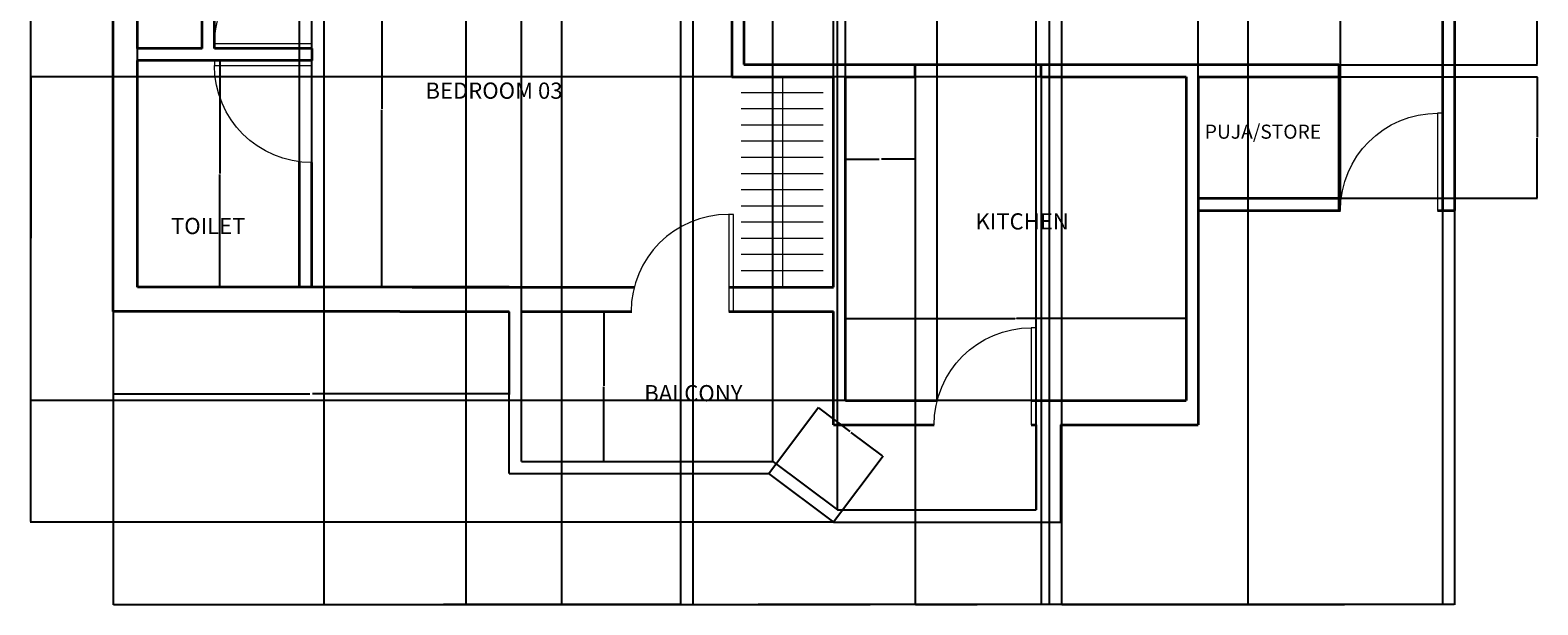
# Model space of a CAD drawing. Units: inches. Extents: x -83 to 475, y -99 to 539.
# Tile 1 of 3: x -83 to 475, y -99 to 114. Entities that reach past the tile are written whole.
import ezdxf

# ---------------------------------------------------------------- set-up
doc = ezdxf.new("R2010")
doc.units = ezdxf.units.IN
doc.header["$LTSCALE"] = 0.5
doc.header["$MEASUREMENT"] = 0
for name, color, linetype, lineweight in [('A-ANNO-DIMS', 2, 'Continuous', 18), ('A-AREA-IDEN', 7, 'Continuous', 18), ('A-DOOR', 3, 'Continuous', 18), ('A-FURN', 8, 'Continuous', 13), ('A-WALL', 7, 'Continuous', 35), ('A-WALL-PRPT', 7, 'Continuous', 25)]:
    doc.layers.add(name, color=color, linetype=linetype, lineweight=lineweight)
doc.styles.get("Standard").update_dxf_attribs({"font": 'arial.ttf'})
doc.dimstyles.get("Standard").update_dxf_attribs({"dimtxt": 0.18, "dimasz": 0.18, "dimexe": 0.18, "dimexo": 0.0625, "dimgap": 0.09, "dimtad": 0, "dimtih": 1, "dimtoh": 1, "dimdec": 4, "dimzin": 0, "dimdsep": 46, "dimtxsty": 'Standard', "dimcen": 0.09, "dimadec": 0, "dimazin": 0, "dimtfac": 1, "dimtdec": 4, "dimtofl": 0, "dimtmove": 0, "dimatfit": 3, "dimfxl": 1, "dimtolj": 1, "dimtzin": 0, "dimarcsym": 0})

# ---------------------------------------------------------------- blocks, each defined once
blk = doc.blocks.new('DOOR-SWING-36')
blk.add_lwpolyline([(1.78, 0), (0, 0), (0, 36.03), (1.78, 36.03)], close=True)
blk.add_arc((1.78, 0), 36, 0, 90)
blk = doc.blocks.new('*D14')
at = {"layer": 'A-ANNO-DIMS', "color": 0, "lineweight": -2, "transparency": 16777216}
for p, q in [((444.04, 47.05), (444.04, -99.07)), ((-52.46, 9.55), (-52.46, -99.07)), ((-52.28, -98.89), (195.39, -98.89)), ((443.86, -98.89), (196.19, -98.89))]:
    blk.add_line(p, q, dxfattribs=at)
at = {"layer": 'A-ANNO-DIMS', "color": 0, "transparency": 16777216}
for points in [[(-52.28, -98.86), (-52.28, -98.92), (-52.46, -98.89)], [(443.86, -98.86), (443.86, -98.92), (444.04, -98.89)]]:
    blk.add_solid(points, dxfattribs=at)
at = {"layer": 'Defpoints', "color": 0, "transparency": 16777216}
for p in [(444.04, 47.11), (-52.46, 9.61), (444.04, -98.89)]:
    blk.add_point(p, dxfattribs=at)
at = {"layer": 'A-ANNO-DIMS', "color": 0, "transparency": 16777216, "insert": (195.79, -98.89), "char_height": 0.18, "attachment_point": 5}
blk.add_mtext('\\A1;496.5', dxfattribs=at)
blk = doc.blocks.new('*D15')
at = {"layer": 'A-ANNO-DIMS', "color": 0, "lineweight": -2, "transparency": 16777216}
for p, q in [((73.48, 492.61), (-83.14, 492.61)), ((-82.96, 492.43), (-82.96, 212.3)), ((-82.96, -68.21), (-82.96, 211.93)), ((214.1, -68.39), (-83.14, -68.39))]:
    blk.add_line(p, q, dxfattribs=at)
at = {"layer": 'A-ANNO-DIMS', "color": 0, "transparency": 16777216}
for points in [[(-82.99, 492.43), (-82.93, 492.43), (-82.96, 492.61)], [(-82.99, -68.21), (-82.93, -68.21), (-82.96, -68.39)]]:
    blk.add_solid(points, dxfattribs=at)
at = {"layer": 'Defpoints', "color": 0, "transparency": 16777216}
for p in [(-82.96, 492.61), (73.54, 492.61), (214.16, -68.39)]:
    blk.add_point(p, dxfattribs=at)
at = {"layer": 'A-ANNO-DIMS', "color": 0, "transparency": 16777216, "insert": (-82.96, 212.11), "char_height": 0.18, "attachment_point": 5}
blk.add_mtext('\\A1;561', dxfattribs=at)
blk = doc.blocks.new('*D16')
at = {"layer": 'A-ANNO-DIMS', "color": 0, "lineweight": -2, "transparency": 16777216}
for p, q in [((78.04, 488.05), (78.04, -99.07)), ((294.04, 488.05), (294.04, -99.07)), ((78.22, -98.89), (185.75, -98.89)), ((293.86, -98.89), (186.33, -98.89))]:
    blk.add_line(p, q, dxfattribs=at)
at = {"layer": 'A-ANNO-DIMS', "color": 0, "transparency": 16777216}
for points in [[(78.22, -98.86), (78.22, -98.92), (78.04, -98.89)], [(293.86, -98.86), (293.86, -98.92), (294.04, -98.89)]]:
    blk.add_solid(points, dxfattribs=at)
at = {"layer": 'Defpoints', "color": 0, "transparency": 16777216}
for p in [(78.04, 488.11), (294.04, 488.11), (294.04, -98.89)]:
    blk.add_point(p, dxfattribs=at)
at = {"layer": 'A-ANNO-DIMS', "color": 0, "transparency": 16777216, "insert": (186.04, -98.89), "char_height": 0.18, "attachment_point": 5}
blk.add_mtext('\\A1;216', dxfattribs=at)
blk = doc.blocks.new('*D19')
at = {"layer": 'A-ANNO-DIMS', "color": 0, "lineweight": -2, "transparency": 16777216}
for p, q in [((25.54, 375.55), (25.54, -99.07)), ((157.54, 375.55), (157.54, -99.07)), ((25.72, -98.89), (91.26, -98.89)), ((157.36, -98.89), (91.82, -98.89))]:
    blk.add_line(p, q, dxfattribs=at)
at = {"layer": 'A-ANNO-DIMS', "color": 0, "transparency": 16777216}
for points in [[(25.72, -98.86), (25.72, -98.92), (25.54, -98.89)], [(157.36, -98.86), (157.36, -98.92), (157.54, -98.89)]]:
    blk.add_solid(points, dxfattribs=at)
at = {"layer": 'Defpoints', "color": 0, "transparency": 16777216}
for p in [(25.54, 375.61), (157.54, 375.61), (157.54, -98.89)]:
    blk.add_point(p, dxfattribs=at)
at = {"layer": 'A-ANNO-DIMS', "color": 0, "transparency": 16777216, "insert": (91.54, -98.89), "char_height": 0.18, "attachment_point": 5}
blk.add_mtext('\\A1;132', dxfattribs=at)
blk = doc.blocks.new('*D20')
at = {"layer": 'A-ANNO-DIMS', "color": 0, "lineweight": -2, "transparency": 16777216}
for p, q in [((162.04, 375.55), (162.04, -99.07)), ((294.04, 357.55), (294.04, -99.07)), ((162.22, -98.89), (227.76, -98.89)), ((293.86, -98.89), (228.32, -98.89))]:
    blk.add_line(p, q, dxfattribs=at)
at = {"layer": 'A-ANNO-DIMS', "color": 0, "transparency": 16777216}
for points in [[(162.22, -98.86), (162.22, -98.92), (162.04, -98.89)], [(293.86, -98.86), (293.86, -98.92), (294.04, -98.89)]]:
    blk.add_solid(points, dxfattribs=at)
at = {"layer": 'Defpoints', "color": 0, "transparency": 16777216}
for p in [(162.04, 375.61), (294.04, 357.61), (294.04, -98.89)]:
    blk.add_point(p, dxfattribs=at)
at = {"layer": 'A-ANNO-DIMS', "color": 0, "transparency": 16777216, "insert": (228.04, -98.89), "char_height": 0.18, "attachment_point": 5}
blk.add_mtext('\\A1;132', dxfattribs=at)
blk = doc.blocks.new('*D27')
at = {"layer": 'A-ANNO-DIMS', "color": 0, "lineweight": -2, "transparency": 16777216}
for p, q in [((367.54, 345.55), (367.54, -99.07)), ((439.54, 345.55), (439.54, -99.07)), ((367.72, -98.89), (403.32, -98.89)), ((439.36, -98.89), (403.76, -98.89))]:
    blk.add_line(p, q, dxfattribs=at)
at = {"layer": 'A-ANNO-DIMS', "color": 0, "transparency": 16777216}
for points in [[(367.72, -98.86), (367.72, -98.92), (367.54, -98.89)], [(439.36, -98.86), (439.36, -98.92), (439.54, -98.89)]]:
    blk.add_solid(points, dxfattribs=at)
at = {"layer": 'Defpoints', "color": 0, "transparency": 16777216}
for p in [(367.54, 345.61), (439.54, 345.61), (439.54, -98.89)]:
    blk.add_point(p, dxfattribs=at)
at = {"layer": 'A-ANNO-DIMS', "color": 0, "transparency": 16777216, "insert": (403.54, -98.89), "char_height": 0.18, "attachment_point": 5}
blk.add_mtext('\\A1;72', dxfattribs=at)
blk = doc.blocks.new('*D33')
at = {"layer": 'A-ANNO-DIMS', "color": 0, "lineweight": -2, "transparency": 16777216}
for p, q in [((25.54, 215.05), (25.54, -99.07)), ((113.54, 215.05), (113.54, -99.07)), ((25.72, -98.89), (69.32, -98.89)), ((113.36, -98.89), (69.76, -98.89))]:
    blk.add_line(p, q, dxfattribs=at)
at = {"layer": 'A-ANNO-DIMS', "color": 0, "transparency": 16777216}
for points in [[(25.72, -98.86), (25.72, -98.92), (25.54, -98.89)], [(113.36, -98.86), (113.36, -98.92), (113.54, -98.89)]]:
    blk.add_solid(points, dxfattribs=at)
at = {"layer": 'Defpoints', "color": 0, "transparency": 16777216}
for p in [(25.54, 215.11), (113.54, 215.11), (113.54, -98.89)]:
    blk.add_point(p, dxfattribs=at)
at = {"layer": 'A-ANNO-DIMS', "color": 0, "transparency": 16777216, "insert": (69.54, -98.89), "char_height": 0.18, "attachment_point": 5}
blk.add_mtext('\\A1;88', dxfattribs=at)
blk = doc.blocks.new('*D35')
at = {"layer": 'A-ANNO-DIMS', "color": 0, "lineweight": -2, "transparency": 16777216}
for p, q in [((21.04, 18.68), (21.04, 523.29)), ((21.22, 523.11), (117.15, 523.11)), ((213.98, 523.11), (118.05, 523.11)), ((214.16, 18.68), (214.16, 523.29))]:
    blk.add_line(p, q, dxfattribs=at)
at = {"layer": 'A-ANNO-DIMS', "color": 0, "transparency": 16777216}
for points in [[(21.22, 523.14), (21.22, 523.08), (21.04, 523.11)], [(213.98, 523.14), (213.98, 523.08), (214.16, 523.11)]]:
    blk.add_solid(points, dxfattribs=at)
at = {"layer": 'Defpoints', "color": 0, "transparency": 16777216}
for p in [(214.16, 523.11), (21.04, 18.61), (214.16, 18.61)]:
    blk.add_point(p, dxfattribs=at)
at = {"layer": 'A-ANNO-DIMS', "color": 0, "transparency": 16777216, "insert": (117.6, 523.11), "char_height": 0.18, "attachment_point": 5}
blk.add_mtext('\\A1;193.12', dxfattribs=at)
blk = doc.blocks.new('*D36')
at = {"layer": 'A-ANNO-DIMS', "color": 0, "lineweight": -2, "transparency": 16777216}
for p, q in [((16.6, 150.61), (47.22, 150.61)), ((47.04, 150.43), (47.04, 84.8)), ((47.04, 18.79), (47.04, 84.43)), ((16.6, 18.61), (47.22, 18.61))]:
    blk.add_line(p, q, dxfattribs=at)
at = {"layer": 'A-ANNO-DIMS', "color": 0, "transparency": 16777216}
for points in [[(47.01, 150.43), (47.07, 150.43), (47.04, 150.61)], [(47.01, 18.79), (47.07, 18.79), (47.04, 18.61)]]:
    blk.add_solid(points, dxfattribs=at)
at = {"layer": 'Defpoints', "color": 0, "transparency": 16777216}
for p in [(16.54, 150.61), (16.54, 18.61), (47.04, 18.61)]:
    blk.add_point(p, dxfattribs=at)
at = {"layer": 'A-ANNO-DIMS', "color": 0, "transparency": 16777216, "insert": (47.04, 84.61), "char_height": 0.18, "attachment_point": 5}
blk.add_mtext('\\A1;132', dxfattribs=at)
blk = doc.blocks.new('*D37')
at = {"layer": 'A-ANNO-DIMS', "color": 0, "lineweight": -2, "transparency": 16777216}
for p, q in [((-43.46, 18.68), (-43.46, 523.29)), ((-43.28, 523.11), (-13.68, 523.11)), ((16.36, 523.11), (-13.24, 523.11)), ((16.54, 18.68), (16.54, 523.29))]:
    blk.add_line(p, q, dxfattribs=at)
at = {"layer": 'A-ANNO-DIMS', "color": 0, "transparency": 16777216}
for points in [[(-43.28, 523.14), (-43.28, 523.08), (-43.46, 523.11)], [(16.36, 523.14), (16.36, 523.08), (16.54, 523.11)]]:
    blk.add_solid(points, dxfattribs=at)
at = {"layer": 'Defpoints', "color": 0, "transparency": 16777216}
for p in [(16.54, 523.11), (-43.46, 18.61), (16.54, 18.61)]:
    blk.add_point(p, dxfattribs=at)
at = {"layer": 'A-ANNO-DIMS', "color": 0, "transparency": 16777216, "insert": (-13.46, 523.11), "char_height": 0.18, "attachment_point": 5}
blk.add_mtext('\\A1;60', dxfattribs=at)
blk = doc.blocks.new('*D38')
at = {"layer": 'A-ANNO-DIMS', "color": 0, "lineweight": -2, "transparency": 16777216}
for p, q in [((-43.4, 102.61), (-12.78, 102.61)), ((-12.96, 102.43), (-12.96, 60.8)), ((-12.96, 18.79), (-12.96, 60.43)), ((-43.4, 18.61), (-12.78, 18.61))]:
    blk.add_line(p, q, dxfattribs=at)
at = {"layer": 'A-ANNO-DIMS', "color": 0, "transparency": 16777216}
for points in [[(-12.99, 102.43), (-12.93, 102.43), (-12.96, 102.61)], [(-12.99, 18.79), (-12.93, 18.79), (-12.96, 18.61)]]:
    blk.add_solid(points, dxfattribs=at)
at = {"layer": 'Defpoints', "color": 0, "transparency": 16777216}
for p in [(-43.46, 102.61), (-43.46, 18.61), (-12.96, 18.61)]:
    blk.add_point(p, dxfattribs=at)
at = {"layer": 'A-ANNO-DIMS', "color": 0, "transparency": 16777216, "insert": (-12.96, 60.61), "char_height": 0.18, "attachment_point": 5}
blk.add_mtext('\\A1;84', dxfattribs=at)
blk = doc.blocks.new('*D39')
at = {"layer": 'A-ANNO-DIMS', "color": 0, "lineweight": -2, "transparency": 16777216}
for p, q in [((218.66, -23.32), (218.66, 7.29)), ((218.84, 7.11), (281.38, 7.11)), ((344.48, 7.11), (281.94, 7.11)), ((344.66, -23.32), (344.66, 7.29))]:
    blk.add_line(p, q, dxfattribs=at)
at = {"layer": 'A-ANNO-DIMS', "color": 0, "transparency": 16777216}
for points in [[(218.84, 7.14), (218.84, 7.08), (218.66, 7.11)], [(344.48, 7.14), (344.48, 7.08), (344.66, 7.11)]]:
    blk.add_solid(points, dxfattribs=at)
at = {"layer": 'Defpoints', "color": 0, "transparency": 16777216}
for p in [(344.66, 7.11), (218.66, -23.39), (344.66, -23.39)]:
    blk.add_point(p, dxfattribs=at)
at = {"layer": 'A-ANNO-DIMS', "color": 0, "transparency": 16777216, "insert": (281.66, 7.11), "char_height": 0.18, "attachment_point": 5}
blk.add_mtext('\\A1;126', dxfattribs=at)
blk = doc.blocks.new('*D40')
at = {"layer": 'A-ANNO-DIMS', "color": 0, "lineweight": -2, "transparency": 16777216}
for p, q in [((344.6, 96.61), (-83.14, 96.61)), ((-82.96, 96.43), (-82.96, 36.8)), ((-82.96, -23.21), (-82.96, 36.43)), ((344.6, -23.39), (-83.14, -23.39))]:
    blk.add_line(p, q, dxfattribs=at)
at = {"layer": 'A-ANNO-DIMS', "color": 0, "transparency": 16777216}
for points in [[(-82.99, 96.43), (-82.93, 96.43), (-82.96, 96.61)], [(-82.99, -23.21), (-82.93, -23.21), (-82.96, -23.39)]]:
    blk.add_solid(points, dxfattribs=at)
at = {"layer": 'Defpoints', "color": 0, "transparency": 16777216}
for p in [(-82.96, 96.61), (344.66, 96.61), (344.66, -23.39)]:
    blk.add_point(p, dxfattribs=at)
at = {"layer": 'A-ANNO-DIMS', "color": 0, "transparency": 16777216, "insert": (-82.96, 36.61), "char_height": 0.18, "attachment_point": 5}
blk.add_mtext('\\A1;120', dxfattribs=at)
blk = doc.blocks.new('*D41')
at = {"layer": 'A-ANNO-DIMS', "color": 0, "lineweight": -2, "transparency": 16777216}
for p, q in [((349.16, 51.68), (349.16, 523.29)), ((349.34, 523.11), (375.13, 523.11)), ((401.58, 523.11), (375.78, 523.11)), ((401.76, 51.68), (401.76, 523.29))]:
    blk.add_line(p, q, dxfattribs=at)
at = {"layer": 'A-ANNO-DIMS', "color": 0, "transparency": 16777216}
for points in [[(349.34, 523.14), (349.34, 523.08), (349.16, 523.11)], [(401.58, 523.14), (401.58, 523.08), (401.76, 523.11)]]:
    blk.add_solid(points, dxfattribs=at)
at = {"layer": 'Defpoints', "color": 0, "transparency": 16777216}
for p in [(401.76, 523.11), (349.16, 51.61), (401.76, 51.61)]:
    blk.add_point(p, dxfattribs=at)
at = {"layer": 'A-ANNO-DIMS', "color": 0, "transparency": 16777216, "insert": (375.46, 523.11), "char_height": 0.18, "attachment_point": 5}
blk.add_mtext('\\A1;52.6', dxfattribs=at)
blk = doc.blocks.new('*D42')
at = {"layer": 'A-ANNO-DIMS', "color": 0, "lineweight": -2, "transparency": 16777216}
for p, q in [((401.22, 96.61), (474.72, 96.61)), ((474.54, 96.43), (474.54, 74.3)), ((474.54, 51.79), (474.54, 73.93)), ((401.82, 51.61), (474.72, 51.61))]:
    blk.add_line(p, q, dxfattribs=at)
at = {"layer": 'A-ANNO-DIMS', "color": 0, "transparency": 16777216}
for points in [[(474.51, 96.43), (474.57, 96.43), (474.54, 96.61)], [(474.51, 51.79), (474.57, 51.79), (474.54, 51.61)]]:
    blk.add_solid(points, dxfattribs=at)
at = {"layer": 'Defpoints', "color": 0, "transparency": 16777216}
for p in [(401.16, 96.61), (474.54, 96.61), (401.76, 51.61)]:
    blk.add_point(p, dxfattribs=at)
at = {"layer": 'A-ANNO-DIMS', "color": 0, "transparency": 16777216, "insert": (474.54, 74.11), "char_height": 0.18, "attachment_point": 5}
blk.add_mtext('\\A1;45', dxfattribs=at)
blk = doc.blocks.new('*D43')
at = {"layer": 'A-ANNO-DIMS', "color": 0, "lineweight": -2, "transparency": 16777216}
for p, q in [((180.98, 101.18), (180.98, 523.29)), ((181.16, 523.11), (309.8, 523.11)), ((439.36, 523.11), (310.73, 523.11)), ((439.54, 83.2), (439.54, 523.29))]:
    blk.add_line(p, q, dxfattribs=at)
at = {"layer": 'A-ANNO-DIMS', "color": 0, "transparency": 16777216}
for points in [[(181.16, 523.14), (181.16, 523.08), (180.98, 523.11)], [(439.36, 523.14), (439.36, 523.08), (439.54, 523.11)]]:
    blk.add_solid(points, dxfattribs=at)
at = {"layer": 'Defpoints', "color": 0, "transparency": 16777216}
for p in [(439.54, 523.11), (180.98, 101.11), (439.54, 83.14)]:
    blk.add_point(p, dxfattribs=at)
at = {"layer": 'A-ANNO-DIMS', "color": 0, "transparency": 16777216, "insert": (310.26, 523.11), "char_height": 0.18, "attachment_point": 5}
blk.add_mtext('\\A1;258.56', dxfattribs=at)
blk = doc.blocks.new('*D44')
at = {"layer": 'A-ANNO-DIMS', "color": 0, "lineweight": -2, "transparency": 16777216}
for p, q in [((439.6, 264.61), (474.72, 264.61)), ((474.54, 264.43), (474.54, 183.05)), ((474.54, 101.29), (474.54, 182.68)), ((401.22, 101.11), (474.72, 101.11))]:
    blk.add_line(p, q, dxfattribs=at)
at = {"layer": 'A-ANNO-DIMS', "color": 0, "transparency": 16777216}
for points in [[(474.51, 264.43), (474.57, 264.43), (474.54, 264.61)], [(474.51, 101.29), (474.57, 101.29), (474.54, 101.11)]]:
    blk.add_solid(points, dxfattribs=at)
at = {"layer": 'Defpoints', "color": 0, "transparency": 16777216}
for p in [(439.54, 264.61), (474.54, 264.61), (401.16, 101.11)]:
    blk.add_point(p, dxfattribs=at)
at = {"layer": 'A-ANNO-DIMS', "color": 0, "transparency": 16777216, "insert": (474.54, 182.86), "char_height": 0.18, "attachment_point": 5}
blk.add_mtext('\\A1;163.5', dxfattribs=at)
blk = doc.blocks.new('*D45')
at = {"layer": 'A-ANNO-DIMS', "color": 0, "lineweight": -2, "transparency": 16777216}
for p, q in [((298.54, 264.55), (298.54, -99.07)), ((439.54, 264.55), (439.54, -99.07)), ((298.72, -98.89), (368.78, -98.89)), ((439.36, -98.89), (369.3, -98.89))]:
    blk.add_line(p, q, dxfattribs=at)
at = {"layer": 'A-ANNO-DIMS', "color": 0, "transparency": 16777216}
for points in [[(298.72, -98.86), (298.72, -98.92), (298.54, -98.89)], [(439.36, -98.86), (439.36, -98.92), (439.54, -98.89)]]:
    blk.add_solid(points, dxfattribs=at)
at = {"layer": 'Defpoints', "color": 0, "transparency": 16777216}
for p in [(298.54, 264.61), (439.54, 264.61), (439.54, -98.89)]:
    blk.add_point(p, dxfattribs=at)
at = {"layer": 'A-ANNO-DIMS', "color": 0, "transparency": 16777216, "insert": (369.04, -98.89), "char_height": 0.18, "attachment_point": 5}
blk.add_mtext('\\A1;141', dxfattribs=at)
blk = doc.blocks.new('*D46')
at = {"layer": 'A-ANNO-DIMS', "color": 0, "lineweight": -2, "transparency": 16777216}
for p, q in [((98.72, 9.61), (129.34, 9.61)), ((129.16, 9.43), (129.16, -17.95)), ((129.16, -45.71), (129.16, -18.32)), ((98.72, -45.89), (129.34, -45.89))]:
    blk.add_line(p, q, dxfattribs=at)
at = {"layer": 'A-ANNO-DIMS', "color": 0, "transparency": 16777216}
for points in [[(129.13, 9.43), (129.19, 9.43), (129.16, 9.61)], [(129.13, -45.71), (129.19, -45.71), (129.16, -45.89)]]:
    blk.add_solid(points, dxfattribs=at)
at = {"layer": 'Defpoints', "color": 0, "transparency": 16777216}
for p in [(98.66, 9.61), (98.66, -45.89), (129.16, -45.89)]:
    blk.add_point(p, dxfattribs=at)
at = {"layer": 'A-ANNO-DIMS', "color": 0, "transparency": 16777216, "insert": (129.16, -18.14), "char_height": 0.18, "attachment_point": 5}
blk.add_mtext('\\A1;55.5', dxfattribs=at)
blk = doc.blocks.new('*D47')
at = {"layer": 'A-ANNO-DIMS', "color": 0, "lineweight": -2, "transparency": 16777216}
for p, q in [((98.66, -45.82), (98.66, 523.29)), ((98.84, 523.11), (144.94, 523.11)), ((191.48, 523.11), (145.38, 523.11)), ((191.66, -45.82), (191.66, 523.29))]:
    blk.add_line(p, q, dxfattribs=at)
at = {"layer": 'A-ANNO-DIMS', "color": 0, "transparency": 16777216}
for points in [[(98.84, 523.14), (98.84, 523.08), (98.66, 523.11)], [(191.48, 523.14), (191.48, 523.08), (191.66, 523.11)]]:
    blk.add_solid(points, dxfattribs=at)
at = {"layer": 'Defpoints', "color": 0, "transparency": 16777216}
for p in [(191.66, 523.11), (98.66, -45.89), (191.66, -45.89)]:
    blk.add_point(p, dxfattribs=at)
at = {"layer": 'A-ANNO-DIMS', "color": 0, "transparency": 16777216, "insert": (145.16, 523.11), "char_height": 0.18, "attachment_point": 5}
blk.add_mtext('\\A1;93', dxfattribs=at)
blk = doc.blocks.new('*D48')
at = {"layer": 'A-ANNO-DIMS', "color": 0, "lineweight": -2, "transparency": 16777216}
for p, q in [((215.66, -63.82), (215.66, 523.29)), ((215.84, 523.11), (252.09, 523.11)), ((288.98, 523.11), (252.73, 523.11)), ((289.16, -63.82), (289.16, 523.29))]:
    blk.add_line(p, q, dxfattribs=at)
at = {"layer": 'A-ANNO-DIMS', "color": 0, "transparency": 16777216}
for points in [[(215.84, 523.14), (215.84, 523.08), (215.66, 523.11)], [(288.98, 523.14), (288.98, 523.08), (289.16, 523.11)]]:
    blk.add_solid(points, dxfattribs=at)
at = {"layer": 'Defpoints', "color": 0, "transparency": 16777216}
for p in [(289.16, 523.11), (215.66, -63.89), (289.16, -63.89)]:
    blk.add_point(p, dxfattribs=at)
at = {"layer": 'A-ANNO-DIMS', "color": 0, "transparency": 16777216, "insert": (252.41, 523.11), "char_height": 0.18, "attachment_point": 5}
blk.add_mtext('\\A1;73.5', dxfattribs=at)
blk = doc.blocks.new('*D49')
at = {"layer": 'A-ANNO-DIMS', "color": 0, "lineweight": -2, "transparency": 16777216}
for p, q in [((190.2, -50.34), (208.57, -25.84)), ((208.6, -26.09), (220.24, -34.82)), ((232.32, -43.88), (220.68, -35.15)), ((214.2, -68.34), (232.57, -43.84))]:
    blk.add_line(p, q, dxfattribs=at)
at = {"layer": 'A-ANNO-DIMS', "color": 0, "transparency": 16777216}
for points in [[(208.62, -26.07), (208.59, -26.12), (208.46, -25.99)], [(232.33, -43.85), (232.3, -43.9), (232.46, -43.99)]]:
    blk.add_solid(points, dxfattribs=at)
at = {"layer": 'Defpoints', "color": 0, "transparency": 16777216}
for p in [(232.46, -43.99), (190.16, -50.39), (214.16, -68.39)]:
    blk.add_point(p, dxfattribs=at)
at = {"layer": 'A-ANNO-DIMS', "color": 0, "transparency": 16777216, "insert": (220.46, -34.99), "char_height": 0.18, "attachment_point": 5}
blk.add_mtext('\\A1;30', dxfattribs=at)
blk = doc.blocks.new('*D50')
at = {"layer": 'A-ANNO-DIMS', "color": 0, "lineweight": -2, "transparency": 16777216}
for p, q in [((-52.46, 9.55), (-52.46, -21.07)), ((94.16, 9.55), (94.16, -21.07)), ((-52.28, -20.89), (20.4, -20.89)), ((93.98, -20.89), (21.3, -20.89))]:
    blk.add_line(p, q, dxfattribs=at)
at = {"layer": 'A-ANNO-DIMS', "color": 0, "transparency": 16777216}
for points in [[(-52.28, -20.86), (-52.28, -20.92), (-52.46, -20.89)], [(93.98, -20.86), (93.98, -20.92), (94.16, -20.89)]]:
    blk.add_solid(points, dxfattribs=at)
at = {"layer": 'Defpoints', "color": 0, "transparency": 16777216}
for p in [(-52.46, 9.61), (94.16, 9.61), (-52.46, -20.89)]:
    blk.add_point(p, dxfattribs=at)
at = {"layer": 'A-ANNO-DIMS', "color": 0, "transparency": 16777216, "insert": (20.85, -20.89), "char_height": 0.18, "attachment_point": 5}
blk.add_mtext('\\A1;146.62', dxfattribs=at)
blk = doc.blocks.new('*D58')
at = {"layer": 'A-ANNO-DIMS', "color": 0, "lineweight": -2, "transparency": 16777216}
for p, q in [((218.66, -23.32), (218.66, 523.29)), ((218.84, 523.11), (235.2, 523.11)), ((252.34, 523.11), (235.98, 523.11)), ((252.52, -23.32), (252.52, 523.29))]:
    blk.add_line(p, q, dxfattribs=at)
at = {"layer": 'A-ANNO-DIMS', "color": 0, "transparency": 16777216}
for points in [[(218.84, 523.14), (218.84, 523.08), (218.66, 523.11)], [(252.34, 523.14), (252.34, 523.08), (252.52, 523.11)]]:
    blk.add_solid(points, dxfattribs=at)
at = {"layer": 'Defpoints', "color": 0, "transparency": 16777216}
for p in [(252.52, 523.11), (218.66, -23.39), (252.52, -23.39)]:
    blk.add_point(p, dxfattribs=at)
at = {"layer": 'A-ANNO-DIMS', "color": 0, "transparency": 16777216, "insert": (235.59, 523.11), "char_height": 0.18, "attachment_point": 5}
blk.add_mtext('\\A1;33.86', dxfattribs=at)
blk = doc.blocks.new('*D59')
at = {"layer": 'A-ANNO-DIMS', "color": 0, "lineweight": -2, "transparency": 16777216}
for p, q in [((218.66, 96.55), (218.66, 65.93)), ((244.35, 96.55), (244.35, 65.93)), ((218.84, 66.11), (231.11, 66.11)), ((244.17, 66.11), (231.9, 66.11))]:
    blk.add_line(p, q, dxfattribs=at)
at = {"layer": 'A-ANNO-DIMS', "color": 0, "transparency": 16777216}
for points in [[(218.84, 66.14), (218.84, 66.08), (218.66, 66.11)], [(244.17, 66.14), (244.17, 66.08), (244.35, 66.11)]]:
    blk.add_solid(points, dxfattribs=at)
at = {"layer": 'Defpoints', "color": 0, "transparency": 16777216}
for p in [(218.66, 96.61), (244.35, 96.61), (218.66, 66.11)]:
    blk.add_point(p, dxfattribs=at)
at = {"layer": 'A-ANNO-DIMS', "color": 0, "transparency": 16777216, "insert": (231.51, 66.11), "char_height": 0.18, "attachment_point": 5}
blk.add_mtext('\\A1;25.69', dxfattribs=at)
blk = doc.blocks.new('*D60')
at = {"layer": 'A-ANNO-DIMS', "color": 0, "lineweight": -2, "transparency": 16777216}
for p, q in [((244.35, 96.55), (244.35, -99.07)), ((291.07, 96.55), (291.07, -99.07)), ((244.53, -98.89), (267.31, -98.89)), ((290.89, -98.89), (268.11, -98.89))]:
    blk.add_line(p, q, dxfattribs=at)
at = {"layer": 'A-ANNO-DIMS', "color": 0, "transparency": 16777216}
for points in [[(244.53, -98.86), (244.53, -98.92), (244.35, -98.89)], [(290.89, -98.86), (290.89, -98.92), (291.07, -98.89)]]:
    blk.add_solid(points, dxfattribs=at)
at = {"layer": 'Defpoints', "color": 0, "transparency": 16777216}
for p in [(244.35, 96.61), (291.07, 96.61), (291.07, -98.89)]:
    blk.add_point(p, dxfattribs=at)
at = {"layer": 'A-ANNO-DIMS', "color": 0, "transparency": 16777216, "insert": (267.71, -98.89), "char_height": 0.18, "attachment_point": 5}
blk.add_mtext('\\A1;46.72', dxfattribs=at)
blk = doc.blocks.new('*D61')
at = {"layer": 'A-ANNO-DIMS', "color": 0, "lineweight": -2, "transparency": 16777216}
for p, q in [((176.48, 96.68), (176.48, 523.29)), ((176.66, 523.11), (194.93, 523.11)), ((213.98, 523.11), (195.71, 523.11)), ((214.16, 96.68), (214.16, 523.29))]:
    blk.add_line(p, q, dxfattribs=at)
at = {"layer": 'A-ANNO-DIMS', "color": 0, "transparency": 16777216}
for points in [[(176.66, 523.14), (176.66, 523.08), (176.48, 523.11)], [(213.98, 523.14), (213.98, 523.08), (214.16, 523.11)]]:
    blk.add_solid(points, dxfattribs=at)
at = {"layer": 'Defpoints', "color": 0, "transparency": 16777216}
for p in [(214.16, 523.11), (176.48, 96.61), (214.16, 96.61)]:
    blk.add_point(p, dxfattribs=at)
at = {"layer": 'A-ANNO-DIMS', "color": 0, "transparency": 16777216, "insert": (195.32, 523.11), "char_height": 0.18, "attachment_point": 5}
blk.add_mtext('\\A1;37.68', dxfattribs=at)

msp = doc.modelspace()

# ---------------------------------------------------------------- linework, layer by layer
at = {"layer": 'A-DOOR'}
for points in [[(21.04, 108.898), (21.04, 107.114), (-14.988, 107.114), (-14.988, 108.898)], [(175.392, 9.614), (177.176, 9.614), (177.176, 45.642), (175.392, 45.642)]]:
    msp.add_lwpolyline(points, close=True, dxfattribs=at)
for centre, end in [((21.04, 108.898), 182.84057), ((175.256, 9.614), 180)]:
    msp.add_arc(centre, 36, 90, end, dxfattribs=at)
at = {"layer": 'A-FURN'}
for p, q in [((195.321, 96.614), (195.321, 18.614)), ((179.946, 90.841), (210.331, 90.841)), ((179.946, 84.841), (210.331, 84.841)), ((179.946, 78.841), (210.331, 78.841)), ((179.946, 72.841), (210.331, 72.841)), ((179.946, 66.841), (210.331, 66.841)), ((179.946, 60.841), (210.331, 60.841)), ((179.946, 54.841), (210.331, 54.841)), ((179.946, 48.841), (210.331, 48.841)), ((179.946, 42.841), (210.331, 42.841)), ((179.946, 36.841), (210.331, 36.841)), ((179.946, 30.841), (210.331, 30.841)), ((179.946, 24.841), (210.331, 24.841))]:
    msp.add_line(p, q, dxfattribs=at)
at = {"layer": 'A-WALL'}
for p, q in [((444.04, 288.614), (444.04, 47.114)), ((-52.46, 9.614), (-52.46, 239.114)), ((439.54, 215.114), (439.54, 47.114)), ((180.981, 155.114), (180.981, 101.114)), ((-43.46, 107.114), (-43.46, 119.114)), ((-19.46, 107.114), (-19.46, 119.114)), ((-14.96, 107.114), (-14.96, 119.114)), ((176.481, 119.086), (176.481, 96.614)), ((-19.46, 107.114), (-43.46, 107.114)), ((21.04, 107.114), (-14.96, 107.114)), ((21.04, 107.114), (21.04, 102.614)), ((-43.46, 18.614), (-43.46, 102.614)), ((21.04, 102.614), (-43.46, 102.614)), ((180.981, 101.114), (401.161, 101.114)), ((244.35, 96.614), (244.35, 101.106)), ((291.071, 96.614), (291.071, 101.081)), ((401.161, 101.114), (401.161, 47.114)), ((176.481, 96.614), (214.161, 96.614)), ((214.161, 18.614), (214.161, 96.614)), ((218.661, -23.386), (218.661, 96.614)), ((218.661, 96.614), (244.35, 96.614)), ((291.071, 96.614), (344.661, 96.614)), ((344.661, 96.614), (344.661, -23.386)), ((349.161, 96.614), (349.161, -32.386)), ((349.161, 96.614), (401.161, 96.614)), ((16.54, 18.614), (16.54, 65.113)), ((16.54, 18.614), (16.54, 65.113)), ((21.04, 18.614), (21.04, 64.83)), ((349.161, 51.614), (401.756, 51.614)), ((349.161, 47.114), (401.756, 47.114)), ((437.756, 47.114), (444.04, 47.114)), ((94.161, 18.614), (-43.46, 18.614)), ((58.161, 18.614), (140.399, 18.614)), ((175.392, 18.614), (177.04, 18.614)), ((175.392, 18.614), (214.161, 18.614)), ((53.661, 9.614), (-52.46, 9.614)), ((53.661, 9.614), (94.161, 9.614)), ((98.661, 9.614), (139.54, 9.614)), ((175.392, 9.614), (177.04, 9.614)), ((175.392, 9.614), (214.161, 9.614)), ((214.161, -32.386), (214.161, 9.614)), ((218.661, -23.386), (252.52, -23.386)), ((287.377, -23.386), (344.661, -23.386)), ((305.756, -23.386), (307.54, -23.386)), ((214.161, -32.386), (251.377, -32.386)), ((287.377, -32.386), (289.161, -32.386)), ((298.161, -32.386), (306.877, -32.386)), ((305.756, -32.386), (349.161, -32.386))]:
    msp.add_line(p, q, dxfattribs=at)
at = {"layer": 'A-WALL-PRPT'}
for p, q in [((94.161, -50.386), (94.161, 9.614)), ((98.661, -45.886), (98.661, 9.614)), ((289.161, -32.386), (289.161, -63.886)), ((298.161, -32.386), (298.161, -68.386)), ((98.661, -45.886), (191.661, -45.886)), ((191.661, -45.886), (215.661, -63.886)), ((94.161, -50.386), (190.161, -50.386)), ((190.161, -50.386), (214.161, -68.386)), ((215.661, -63.886), (289.161, -63.886)), ((214.161, -68.386), (298.161, -68.386))]:
    msp.add_line(p, q, dxfattribs=at)

# ---------------------------------------------------------------- block references
at = {"layer": 'A-DOOR', "extrusion": (0, 0, -1), "zscale": -1, "rotation": 270}
msp.add_blockref('DOOR-SWING-36', (-21.04, 102.614), dxfattribs=at)
at = {"layer": 'A-DOOR', "extrusion": (0, 0, -1), "zscale": -1}
for p in [(-439.54, 47.114), (-289.161, -32.386)]:
    msp.add_blockref('DOOR-SWING-36', p, dxfattribs=at)

# ---------------------------------------------------------------- texts
at = {"layer": 'A-AREA-IDEN'}
for s, height, p in [('BEDROOM 03', 6, (63.144, 88.485)), ('PUJA/STORE', 5.2166, (351.577, 73.674)), ('KITCHEN', 6, (266.737, 40.039)), ('TOILET', 6, (-31.039, 38.333)), ('BALCONY', 6, (144.117, -23.611))]:
    msp.add_text(s, height=height, dxfattribs=at).set_placement(p)

# ---------------------------------------------------------------- dimensions: what is measured, and where the dimension line sits
at = {"layer": 'A-ANNO-DIMS'}
for base, p1, p2, override, picture, middle in [((16.54, 523.114), (-43.46, 18.614), (16.54, 18.614), {"dimdec": 0, "dimlfac": 1, "dimrnd": 0, "dimzin": 0, "dimdsep": 46, "dimlunit": 2}, '*D37', (-13.46, 523.114)), ((214.161, 523.114), (21.04, 18.614), (214.161, 18.614), {"dimdec": 2, "dimlfac": 1, "dimrnd": 0, "dimzin": 0, "dimdsep": 46, "dimlunit": 2}, '*D35', (117.601, 523.114)), ((191.661, 523.114), (98.661, -45.886), (191.661, -45.886), {"dimdec": 0, "dimlfac": 1, "dimrnd": 0, "dimzin": 0, "dimdsep": 46, "dimlunit": 2}, '*D47', (145.161, 523.114)), ((214.161, 523.114), (176.481, 96.614), (214.161, 96.614), {"dimdec": 2, "dimlfac": 1, "dimrnd": 0, "dimzin": 0, "dimdsep": 46, "dimlunit": 2}, '*D61', (195.321, 523.114)), ((439.54, 523.114), (180.981, 101.114), (439.54, 83.142), {"dimdec": 2, "dimlfac": 1, "dimrnd": 0, "dimzin": 0, "dimdsep": 46, "dimlunit": 2}, '*D43', (310.26, 523.114)), ((289.161, 523.114), (215.661, -63.886), (289.161, -63.886), {"dimdec": 1, "dimlfac": 1, "dimrnd": 0, "dimzin": 0, "dimdsep": 46, "dimlunit": 2}, '*D48', (252.411, 523.114)), ((252.52, 523.114), (218.661, -23.386), (252.52, -23.386), {"dimdec": 2, "dimlfac": 1, "dimrnd": 0, "dimzin": 0, "dimdsep": 46, "dimlunit": 2}, '*D58', (235.591, 523.114)), ((401.756, 523.114), (349.161, 51.614), (401.756, 51.614), {"dimdec": 1, "dimlfac": 1, "dimrnd": 0, "dimzin": 0, "dimdsep": 46, "dimlunit": 2}, '*D41', (375.459, 523.114)), ((294.04, -98.886), (78.04, 488.114), (294.04, 488.114), {"dimdec": 0, "dimlfac": 1, "dimrnd": 0, "dimzin": 0, "dimdsep": 46, "dimlunit": 2}, '*D16', (186.04, -98.886)), ((157.54, -98.886), (25.54, 375.614), (157.54, 375.614), {"dimdec": 0, "dimlfac": 1, "dimrnd": 0, "dimzin": 0, "dimdsep": 46, "dimlunit": 2}, '*D19', (91.54, -98.886)), ((294.04, -98.886), (162.04, 375.614), (294.04, 357.614), {"dimdec": 0, "dimlfac": 1, "dimrnd": 0, "dimzin": 0, "dimdsep": 46, "dimlunit": 2}, '*D20', (228.04, -98.886)), ((439.54, -98.886), (367.54, 345.614), (439.54, 345.614), {"dimdec": 0, "dimlfac": 1, "dimrnd": 0, "dimzin": 0, "dimdsep": 46, "dimlunit": 2}, '*D27', (403.54, -98.886)), ((439.54, -98.886), (298.54, 264.614), (439.54, 264.614), {"dimdec": 0, "dimlfac": 1, "dimrnd": 0, "dimzin": 0, "dimdsep": 46, "dimlunit": 2}, '*D45', (369.04, -98.886)), ((113.54, -98.886), (25.54, 215.114), (113.54, 215.114), {"dimdec": 0, "dimlfac": 1, "dimrnd": 0, "dimzin": 0, "dimdsep": 46, "dimlunit": 2}, '*D33', (69.54, -98.886)), ((291.071, -98.886), (244.35, 96.614), (291.071, 96.614), {"dimdec": 2, "dimlfac": 1, "dimrnd": 0, "dimzin": 0, "dimdsep": 46, "dimlunit": 2}, '*D60', (267.711, -98.886)), ((444.04, -98.886), (-52.46, 9.614), (444.04, 47.114), {"dimdec": 1, "dimlfac": 1, "dimrnd": 0, "dimzin": 0, "dimdsep": 46, "dimlunit": 2}, '*D14', (195.79, -98.886)), ((344.661, 7.114), (218.661, -23.386), (344.661, -23.386), {"dimdec": 0, "dimlfac": 1, "dimrnd": 0, "dimzin": 0, "dimdsep": 46, "dimlunit": 2}, '*D39', (281.661, 7.114))]:
    dim = msp.add_linear_dim(base=base, p1=p1, p2=p2, dimstyle='Standard', override=override, dxfattribs=at)
    dim.commit()
    dim.dimension.update_dxf_attribs({"geometry": picture, "text_midpoint": middle})
for base, p1, p2, angle, override, picture, middle in [((-82.96, 492.614), (214.161, -68.386), (73.54, 492.614), 90, {"dimdec": 0, "dimlfac": 1, "dimrnd": 0, "dimzin": 0, "dimdsep": 46, "dimlunit": 2}, '*D15', (-82.96, 212.114)), ((474.54, 264.614), (401.161, 101.114), (439.54, 264.614), 90, {"dimdec": 1, "dimlfac": 1, "dimrnd": 0, "dimzin": 0, "dimdsep": 46, "dimlunit": 2}, '*D44', (474.54, 182.864)), ((47.04, 18.614), (16.54, 150.614), (16.54, 18.614), 270, {"dimdec": 0, "dimlfac": 1, "dimrnd": 0, "dimzin": 0, "dimdsep": 46, "dimlunit": 2}, '*D36', (47.04, 84.614)), ((-12.96, 18.614), (-43.46, 102.614), (-43.46, 18.614), 270, {"dimdec": 0, "dimlfac": 1, "dimrnd": 0, "dimzin": 0, "dimdsep": 46, "dimlunit": 2}, '*D38', (-12.96, 60.614)), ((-82.96, 96.614), (344.661, -23.386), (344.661, 96.614), 90, {"dimdec": 0, "dimlfac": 1, "dimrnd": 0, "dimzin": 0, "dimdsep": 46, "dimlunit": 2}, '*D40', (-82.96, 36.614)), ((218.661, 66.114), (244.35, 96.614), (218.661, 96.614), 180, {"dimdec": 2, "dimlfac": 1, "dimrnd": 0, "dimzin": 0, "dimdsep": 46, "dimlunit": 2}, '*D59', (231.506, 66.114)), ((474.54, 96.614), (401.756, 51.614), (401.161, 96.614), 90, {"dimdec": 0, "dimlfac": 1, "dimrnd": 0, "dimzin": 0, "dimdsep": 46, "dimlunit": 2}, '*D42', (474.54, 74.114)), ((-52.46, -20.886), (94.161, 9.614), (-52.46, 9.614), 180, {"dimdec": 2, "dimlfac": 1, "dimrnd": 0, "dimzin": 0, "dimdsep": 46, "dimlunit": 2}, '*D50', (20.851, -20.886)), ((129.161, -45.886), (98.661, 9.614), (98.661, -45.886), 270, {"dimdec": 1, "dimlfac": 1, "dimrnd": 0, "dimzin": 0, "dimdsep": 46, "dimlunit": 2}, '*D46', (129.161, -18.136)), ((232.461, -43.986), (190.161, -50.386), (214.161, -68.386), 323.1301, {"dimdec": 0, "dimlfac": 1, "dimrnd": 0, "dimzin": 0, "dimdsep": 46, "dimlunit": 2}, '*D49', (220.461, -34.986))]:
    dim = msp.add_linear_dim(base=base, p1=p1, p2=p2, angle=angle, dimstyle='Standard', override=override, dxfattribs=at)
    dim.commit()
    dim.dimension.update_dxf_attribs({"geometry": picture, "text_midpoint": middle})

doc.saveas('drawing.dxf')
